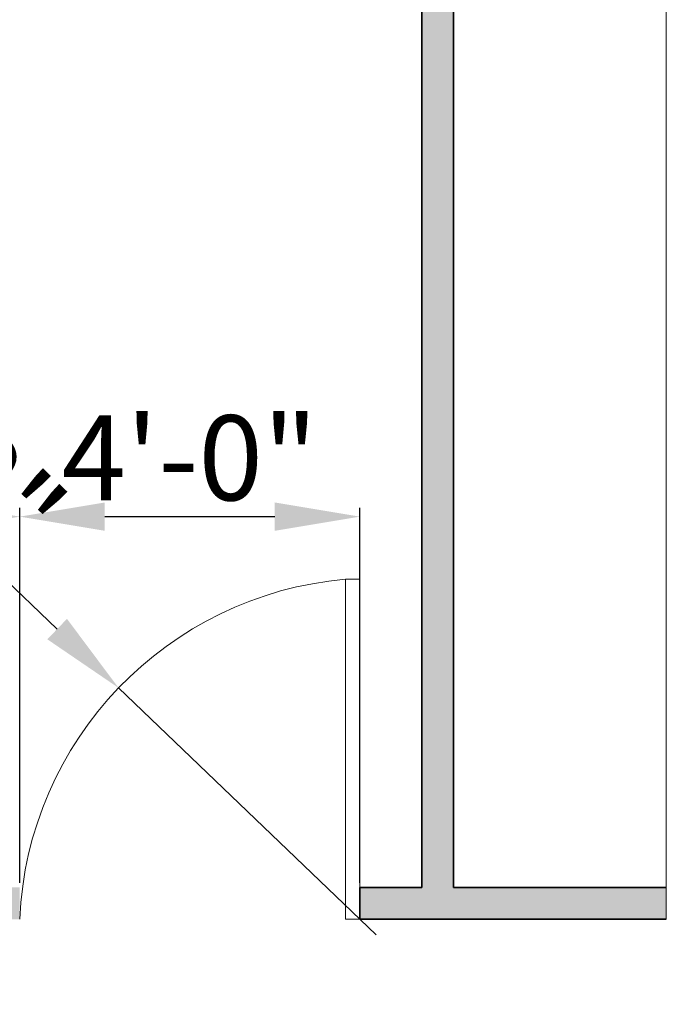
# Model space of a CAD drawing. Units: inches. Extents: x 2083 to 3317, y 1141 to 2115.
# Tile 103 of 256: x 2415 to 2508, y 1794 to 1933. Entities that reach past the tile are written whole.
import ezdxf

# ---------------------------------------------------------------- set-up
doc = ezdxf.new("R2010")
doc.units = ezdxf.units.IN
for name, color, linetype, lineweight in [('A-ANNO-DIMS', 2, 'Continuous', 18), ('A-DOOR', 4, 'Continuous', 18), ('A-FLOR-CASE', 8, 'Continuous', 18), ('A-WALL', 7, 'Continuous', 35)]:
    doc.layers.add(name, color=color, linetype=linetype, lineweight=lineweight)
doc.layers.add('A-WALL-PATT', color=251, linetype='Continuous', lineweight=13, true_color=0x636466)
doc.styles.get("Standard").update_dxf_attribs({"font": 'arial.ttf'})
doc.dimstyles.new('ISO-25', dxfattribs={"dimtxt": 12, "dimasz": 12, "dimexe": 1.25, "dimexo": 0.625, "dimtad": 1, "dimlunit": 3, "dimtxsty": 'Standard', "dimcen": 2.5, "dimadec": 0, "dimazin": 0, "dimtfac": 1, "dimtmove": 0, "dimatfit": 3, "dimfxl": 1, "dimarcsym": 0})

# ---------------------------------------------------------------- blocks, each defined once
blk = doc.blocks.new('*D53')
at = {"layer": 'A-ANNO-DIMS', "color": 0, "lineweight": -2, "transparency": 16777216}
for p, q in [((2235.96, 1810.64), (2235.96, 1863.61)), ((2414.72, 1810.64), (2414.72, 1863.61)), ((2247.96, 1862.36), (2402.72, 1862.36))]:
    blk.add_line(p, q, dxfattribs=at)
at = {"layer": 'A-ANNO-DIMS', "color": 0, "transparency": 16777216}
for points in [[(2247.96, 1864.36), (2247.96, 1860.36), (2235.96, 1862.36)], [(2402.72, 1864.36), (2402.72, 1860.36), (2414.72, 1862.36)]]:
    blk.add_solid(points, dxfattribs=at)
at = {"layer": 'Defpoints', "color": 0, "transparency": 16777216}
for p in [(2414.72, 1862.36), (2235.96, 1810.01), (2414.72, 1810.01)]:
    blk.add_point(p, dxfattribs=at)
at = {"layer": 'A-ANNO-DIMS', "color": 0, "transparency": 16777216, "insert": (2325.34, 1869.01), "char_height": 12, "attachment_point": 5}
blk.add_mtext('14\'-11"', dxfattribs=at)
blk = doc.blocks.new('*D54')
at = {"layer": 'A-ANNO-DIMS', "color": 0, "lineweight": -2, "transparency": 16777216}
for p, q in [((2414.72, 1810.64), (2414.72, 1863.61)), ((2462.72, 1810.64), (2462.72, 1863.61)), ((2426.72, 1862.36), (2450.72, 1862.36))]:
    blk.add_line(p, q, dxfattribs=at)
at = {"layer": 'A-ANNO-DIMS', "color": 0, "transparency": 16777216}
for points in [[(2426.72, 1864.36), (2426.72, 1860.36), (2414.72, 1862.36)], [(2450.72, 1864.36), (2450.72, 1860.36), (2462.72, 1862.36)]]:
    blk.add_solid(points, dxfattribs=at)
at = {"layer": 'Defpoints', "color": 0, "transparency": 16777216}
for p in [(2462.72, 1862.36), (2414.72, 1810.01), (2462.72, 1810.01)]:
    blk.add_point(p, dxfattribs=at)
at = {"layer": 'A-ANNO-DIMS', "color": 0, "transparency": 16777216, "insert": (2438.72, 1869.11), "char_height": 12, "attachment_point": 5}
blk.add_mtext('4\'-0"', dxfattribs=at)
blk = doc.blocks.new('*D68')
at = {"layer": 'A-ANNO-DIMS', "color": 0, "lineweight": -2, "transparency": 16777216}
for p, q in [((2358.93, 1905.02), (2420.01, 1846.48)), ((2465.03, 1803.34), (2428.67, 1838.18))]:
    blk.add_line(p, q, dxfattribs=at)
at = {"layer": 'A-ANNO-DIMS', "color": 0, "transparency": 16777216}
blk.add_solid([(2421.39, 1847.93), (2418.62, 1845.04), (2428.67, 1838.18)], dxfattribs=at)
at = {"layer": 'Defpoints', "color": 0, "transparency": 16777216}
for p in [(2428.67, 1838.18), (2465.03, 1803.34)]:
    blk.add_point(p, dxfattribs=at)
at = {"layer": 'A-ANNO-DIMS', "color": 0, "transparency": 16777216, "insert": (2389.86, 1884.83), "char_height": 12, "attachment_point": 5, "rotation": 316.2184}
blk.add_mtext('R4\'-2 1/2"', dxfattribs=at)

msp = doc.modelspace()

# ---------------------------------------------------------------- hatches: boundary and pattern name
at = {"layer": 'A-WALL-PATT'}
h = msp.add_hatch(color=256, dxfattribs=at)
h.dxf.hatch_style = 1
h.paths.add_polyline_path([(3126.96, 2020.761), (2748.96, 2020.761), (2604.96, 2020.761), (2226.96, 2020.761), (2226.96, 1702.761), (2466.96, 1702.761), (2466.96, 1582.761), (2418.96, 1582.761), (2418.96, 1477.761), (2226.96, 1477.761), (2226.96, 1263.261), (2544.96, 1263.261), (2544.96, 1411.761), (2604.96, 1411.761), (2685.96, 1411.761), (2685.96, 1420.761), (2604.96, 1420.761), (2604.96, 1573.761), (2604.96, 1702.761), (2604.96, 2011.761), (2748.96, 2011.761), (2748.96, 1702.761), (2862.96, 1702.761), (2862.96, 1621.761), (2871.96, 1621.761), (2871.96, 1702.761), (2883.96, 1702.761), (2883.96, 1706.939, -0.0264593), (2883.96, 1711.761), (2757.96, 1711.761), (2757.96, 1807.761), (2787.96, 1807.761), (2787.96, 1812.261), (2757.96, 1812.261), (2757.96, 2011.761), (2877.96, 2011.761), (2877.96, 1812.261), (2847.96, 1812.261), (2847.96, 1807.761), (2889.836, 1807.761), (2889.836, 1812.261), (2882.46, 1812.261), (2882.46, 2011.761), (3117.96, 2011.761), (3117.96, 1812.261), (2937.836, 1812.261), (2937.836, 1807.761), (2995.71, 1807.761), (2995.71, 1796.118), (3000.21, 1796.118), (3000.21, 1807.761), (3117.96, 1807.761), (3117.96, 1711.761), (3000.21, 1711.761), (3000.21, 1760.118), (2998.573, 1760.118, -0.020711), (2995.71, 1760.118), (2995.71, 1711.761), (2931.96, 1711.761), (2931.96, 1702.761), (3126.96, 1702.761)])
h.paths.add_polyline_path([(2471.46, 2011.761), (2471.46, 1810.011), (2462.717, 1810.011), (2462.717, 1805.511), (2505.96, 1805.511), (2505.96, 1810.011), (2475.96, 1810.011), (2475.96, 2011.761), (2595.96, 2011.761), (2595.96, 1810.011), (2565.96, 1810.011), (2565.96, 1805.511), (2595.96, 1805.511), (2595.96, 1711.761), (2235.96, 1711.761), (2235.96, 1805.511), (2353.71, 1805.511), (2353.71, 1796.054), (2358.21, 1796.054), (2358.21, 1805.511), (2414.717, 1805.511), (2414.717, 1810.011), (2235.96, 1810.011), (2235.96, 2011.761)], flags=16)
h.paths.add_polyline_path([(2270.205, 1994.61), (2270.205, 1970.61), (2246.205, 1970.61), (2246.205, 1994.61)], flags=0)
edge = h.paths.add_edge_path(flags=0)
edge.add_ellipse((2332.027, 1899.798), major_axis=(-3.043, 3.043), ratio=0.1682525, start_angle=-161.33217, end_angle=-156.30711, ccw=False)
edge.add_ellipse((2333.082, 1898.744), major_axis=(-1.055, 1.055), ratio=0.4535321, start_angle=-123.37102, end_angle=-94.15911)
edge = h.paths.add_edge_path(flags=0)
edge.add_ellipse((2332.027, 1968.876), major_axis=(3.043, 3.043), ratio=0.1682525, start_angle=18.66783, end_angle=23.69289)
edge.add_spline(control_points=[(2332.926, 1970.691), (2332.227, 1970.336), (2330.894, 1969.659), (2328.413, 1970.932), (2327.204, 1967.749), (2324.71, 1969.956), (2322.533, 1967.012), (2320.013, 1971.296), (2317.68, 1968.158), (2316.041, 1967.102), (2315.427, 1966.81)], knot_values=[0, 0, 0, 0, 2.2670587, 4.3245589, 6.6855835, 8.8786411, 11.121502, 14.300359, 17.7552837, 19.732645, 19.732645, 19.732645, 19.732645], degree=3, periodic=0)
edge.add_ellipse((2332.027, 1968.876), major_axis=(3.043, 3.043), ratio=0.1682525, start_angle=18.66783, end_angle=23.69289, ccw=False)
edge.add_ellipse((2333.082, 1969.931), major_axis=(1.055, 1.055), ratio=0.4535321, start_angle=56.62898, end_angle=85.84089, ccw=False)
edge = h.paths.add_edge_path(flags=0)
edge.add_spline(control_points=[(2296.428, 1967.988), (2293.628, 1965.336), (2287.704, 1959.727), (2299.744, 1949.996), (2294.533, 1935.669), (2290.573, 1920.604), (2293.394, 1909.974), (2296.185, 1904.967)], knot_values=[0.0991853, 0.0991853, 0.0991853, 0.0991853, 0.3453009, 0.6198217, 0.9826526, 1.3860932, 1.8105546, 1.8105546, 1.8105546, 1.8105546], degree=3, periodic=0)
edge.add_spline(control_points=[(2296.185, 1904.967), (2297.384, 1902.619), (2298.001, 1901.949), (2298.553, 1901.468)], knot_values=[0.0062457, 0.0062457, 0.0062457, 0.0062457, 0.0554759, 0.0554759, 0.0554759, 0.0554759], degree=3, periodic=0)
edge.add_spline(control_points=[(2298.553, 1901.468), (2297.259, 1900.923), (2295.225, 1900.232), (2293.06, 1900.614), (2292.101, 1900.788), (2292.09, 1900.791)], knot_values=[0.3128349, 0.3128349, 0.3128349, 0.3128349, 0.4017797, 0.4749867, 0.4759027, 0.4759027, 0.4759027, 0.4759027], degree=3, periodic=0)
edge.add_arc((2292.794, 1904.664), 3.937, 215.4209, 259.69818, ccw=False)
edge.add_spline(control_points=[(2289.585, 1902.382), (2289.477, 1902.535), (2289.368, 1902.688), (2289.261, 1902.841)], knot_values=[0.1028719, 0.1028719, 0.1028719, 0.1028719, 0.1168958, 0.1168958, 0.1168958, 0.1168958], degree=3, periodic=0)
edge.add_spline(control_points=[(2289.261, 1902.841), (2288.687, 1902.55), (2287.64, 1902.02), (2285.881, 1901.874), (2283.853, 1901.504), (2281.72, 1899.711), (2278.467, 1899.493), (2276.157, 1901.883), (2272.259, 1899.804), (2267.778, 1901.843), (2262.244, 1900.184), (2257.415, 1901.782), (2254.318, 1900.726), (2253.178, 1900.337)], knot_values=[0, 0, 0, 0, 1.9079767, 3.4771759, 5.261074, 7.9728515, 11.6802485, 13.7179214, 16.9395917, 22.789562, 27.5025027, 33.5952153, 37.1456181, 37.1456181, 37.1456181, 37.1456181], degree=3, periodic=0)
edge.add_line((2253.178, 1900.337), (2250.244, 1902.841))
edge.add_line((2250.244, 1902.841), (2250.244, 1965.833))
edge.add_line((2250.244, 1965.833), (2253.178, 1968.337))
edge.add_spline(control_points=[(2253.178, 1968.337), (2254.318, 1967.948), (2257.415, 1966.892), (2262.244, 1968.49), (2267.778, 1966.831), (2271.527, 1968.537), (2273.876, 1967.828), (2274.207, 1967.728)], knot_values=[0, 0, 0, 0, 0.0901802, 0.2449351, 0.3646438, 0.5132331, 0.5378548, 0.5378548, 0.5378548, 0.5378548], degree=3, periodic=0)
edge.add_arc((2274.353, 1963.793), 3.937, 72.05113, 92.12795, ccw=False)
edge.add_arc((2281.297, 1985.23), 18.596, 252.05113, 288.56572)
edge.add_arc((2292.317, 1956.029), 12.646, 71.02679, 113.77822, ccw=False)
edge = h.paths.add_edge_path(flags=0)
edge.add_spline(control_points=[(2274.899, 1951.856), (2275.066, 1951.617), (2275.233, 1951.377), (2275.398, 1951.136)], knot_values=[1.4099157, 1.4099157, 1.4099157, 1.4099157, 1.4315903, 1.4315903, 1.4315903, 1.4315903], degree=3, periodic=0)
edge.add_spline(control_points=[(2275.398, 1951.136), (2275.792, 1950.562), (2276.179, 1949.984), (2276.546, 1949.397)], knot_values=[1.3582378, 1.3582378, 1.3582378, 1.3582378, 1.4099157, 1.4099157, 1.4099157, 1.4099157], degree=3, periodic=0)
edge.add_line((2276.546, 1949.397), (2277.437, 1947.862))
edge.add_spline(control_points=[(2277.437, 1947.862), (2276.304, 1945.673), (2274.64, 1942.427), (2274.632, 1938.094), (2272.799, 1930.852), (2274.356, 1943.897), (2275.948, 1947.923), (2276.546, 1949.397)], knot_values=[0.0056315, 0.0056315, 0.0056315, 0.0056315, 0.1860139, 0.2660015, 0.3570872, 0.5963902, 0.7397317, 0.7397317, 0.7397317, 0.7397317], degree=3, periodic=0)
edge.add_spline(control_points=[(2276.546, 1949.397), (2276.179, 1949.984), (2275.792, 1950.562), (2275.398, 1951.136)], knot_values=[1.3582378, 1.3582378, 1.3582378, 1.3582378, 1.4099157, 1.4099157, 1.4099157, 1.4099157], degree=3, periodic=0)
edge.add_spline(control_points=[(2275.398, 1951.136), (2274.943, 1950.08), (2274.208, 1948.025), (2273.935, 1944.851), (2272.469, 1937.627), (2273.466, 1945.696), (2274.701, 1951.059), (2274.899, 1951.856)], knot_values=[0.1043639, 0.1043639, 0.1043639, 0.1043639, 0.1896363, 0.2696239, 0.3607096, 0.6000126, 0.6446217, 0.6446217, 0.6446217, 0.6446217], degree=3, periodic=0)
h.paths.add_polyline_path([(2269.168, 1963.128, -0.3575267), (2268.171, 1960.976, -0.0925607), (2268.171, 1939.436, -0.3575267), (2269.168, 1937.285, -0.3575267), (2267.016, 1938.282, -0.1647847), (2254.686, 1938.282, -0.3575267), (2252.534, 1937.285, -0.3575267), (2253.531, 1939.436, -0.0925607), (2253.531, 1960.976, -0.3575267), (2252.534, 1963.128, -0.3575267), (2254.686, 1962.131, -0.1647847), (2267.016, 1962.131, -0.3575267)], flags=0)
h.paths.add_polyline_path([(2248.874, 1967.802), (2248.874, 1957.028), (2249.458, 1957.028), (2249.458, 1911.647), (2248.874, 1911.647), (2248.874, 1900.873), (2246.512, 1900.873, 0.1973271), (2244.15, 1902.457), (2244.15, 1966.218, 0.1973271), (2246.512, 1967.802)], flags=0)
h.paths.add_polyline_path([(2269.168, 1931.389, -0.3575267), (2268.171, 1929.238, -0.0925607), (2268.171, 1907.698, -0.3575267), (2269.168, 1905.547, -0.3575267), (2267.016, 1906.544, -0.1647847), (2254.686, 1906.544, -0.3575267), (2252.534, 1905.547, -0.3575267), (2253.531, 1907.698, -0.0925607), (2253.531, 1929.238, -0.3575267), (2252.534, 1931.389, -0.3575267), (2254.686, 1930.392, -0.1647847), (2267.016, 1930.392, -0.3575267)], flags=0)
edge = h.paths.add_edge_path(flags=0)
edge.add_spline(control_points=[(2276.197, 1906.724), (2276.168, 1909.029), (2276.114, 1913.372), (2270.598, 1924.925), (2273.905, 1919.013), (2275.922, 1916.262), (2275.475, 1912.402), (2277.258, 1910.381), (2276.696, 1908.225), (2276.646, 1906.813), (2276.618, 1906.008)], knot_values=[0, 0, 0, 0, 8.6102597, 16.2212739, 18.8430575, 23.8048978, 27.4408283, 29.3561016, 31.2034776, 33.6506866, 33.6506866, 33.6506866, 33.6506866], degree=3, periodic=0)
edge.add_spline(control_points=[(2276.618, 1906.008), (2276.623, 1905.624), (2276.498, 1904.629), (2275.442, 1903.855), (2274.937, 1903.08), (2274.859, 1902.841)], knot_values=[0.1564884, 0.1564884, 0.1564884, 0.1564884, 0.1843975, 0.2313765, 0.2505985, 0.2505985, 0.2505985, 0.2505985], degree=3, periodic=0)
edge.add_line((2274.859, 1902.841), (2276.506, 1902.841))
edge.add_spline(control_points=[(2276.506, 1902.841), (2276.788, 1903.085), (2277.665, 1904.125), (2278.25, 1904.341), (2277.654, 1908.527), (2278.156, 1906.228), (2278.1, 1905.286), (2278.847, 1904.069), (2277.857, 1903.415), (2277.874, 1902.991), (2277.904, 1902.841)], knot_values=[0.0595743, 0.0595743, 0.0595743, 0.0595743, 0.0807529, 0.1037415, 0.1697201, 0.1760361, 0.2071372, 0.2404744, 0.2623409, 0.2736605, 0.2736605, 0.2736605, 0.2736605], degree=3, periodic=0)
edge.add_line((2277.904, 1902.841), (2280.03, 1902.841))
edge.add_spline(control_points=[(2280.03, 1902.841), (2279.888, 1903.088), (2279.499, 1903.982), (2280.152, 1905.939), (2278.104, 1909.658), (2279.762, 1907.185), (2280.328, 1904.875), (2280.485, 1903.49), (2281.463, 1903.249), (2281.758, 1902.936), (2281.834, 1902.841)], knot_values=[0.013856, 0.013856, 0.013856, 0.013856, 0.0348738, 0.0888667, 0.1078792, 0.1267378, 0.158714, 0.1937575, 0.2174868, 0.2267221, 0.2267221, 0.2267221, 0.2267221], degree=3, periodic=0)
edge.add_spline(control_points=[(2281.834, 1902.841), (2281.788, 1902.827), (2281.647, 1902.783), (2281.396, 1902.859), (2281.088, 1902.985), (2280.721, 1903.061), (2280.333, 1903.026), (2280.125, 1902.899), (2280.03, 1902.841)], knot_values=[0, 0, 0, 0, 0.1441304, 0.435517, 0.7492759, 1.1530457, 1.5483707, 1.878348, 1.878348, 1.878348, 1.878348], degree=3, periodic=0)
edge.add_line((2280.03, 1902.841), (2277.904, 1902.841))
edge.add_spline(control_points=[(2277.904, 1902.841), (2277.893, 1902.796), (2277.865, 1902.68), (2277.607, 1902.687), (2277.274, 1902.801), (2276.838, 1902.62), (2276.584, 1902.789), (2276.506, 1902.841)], knot_values=[0, 0, 0, 0, 0.1271885, 0.3261988, 0.6280094, 1.2435704, 1.5153306, 1.5153306, 1.5153306, 1.5153306], degree=3, periodic=0)
edge.add_line((2276.506, 1902.841), (2274.859, 1902.841))
edge.add_spline(control_points=[(2274.859, 1902.841), (2274.814, 1902.899), (2274.725, 1903.013), (2274.493, 1903.119), (2274.244, 1902.961), (2273.937, 1903.185), (2273.614, 1902.983), (2273.408, 1902.883), (2273.322, 1902.841)], knot_values=[0, 0, 0, 0, 0.2184302, 0.4369566, 0.6879766, 0.9903786, 1.3983955, 1.6918498, 1.6918498, 1.6918498, 1.6918498], degree=3, periodic=0)
edge.add_spline(control_points=[(2273.322, 1902.841), (2273.617, 1903.446), (2274.274, 1904.538), (2276.027, 1904.574), (2276.207, 1906.584), (2276.197, 1906.724)], knot_values=[0.0122268, 0.0122268, 0.0122268, 0.0122268, 0.0594721, 0.1062177, 0.134458, 0.134458, 0.134458, 0.134458], degree=3, periodic=0)
h.paths.add_polyline_path([(2270.776, 1897.79), (2270.776, 1873.79), (2246.776, 1873.79), (2246.776, 1897.79)], flags=0)
h.paths.add_polyline_path([(2353.71, 1760.005), (2353.71, 1760.054), (2358.21, 1760.054, -0.033729)], flags=0)
h.paths.add_polyline_path([(2321.819, 1737.529), (2341.995, 1737.529, -0.4142136), (2343.203, 1736.321), (2343.203, 1721.021, -0.4142136), (2341.995, 1719.813), (2321.819, 1719.813, -0.4142136), (2320.611, 1721.021), (2320.611, 1736.321, -0.4142136)], flags=0)
h.paths.add_polyline_path([(2324.235, 1736.321), (2339.579, 1736.321, -0.4142136), (2341.995, 1733.905), (2341.995, 1725.45, -0.4142136), (2339.579, 1723.034), (2333.681, 1723.034), (2333.845, 1722.045, -0.8706461), (2335.425, 1721.826, -0.767327), (2333.923, 1721.423), (2331.291, 1721.423, -0.767327), (2329.788, 1721.826, -0.8706461), (2331.368, 1722.045), (2331.533, 1723.034), (2324.235, 1723.034, -0.4142136), (2321.819, 1725.45), (2321.819, 1733.905, -0.4142136)], flags=0)
h.paths.add_polyline_path([(2570.484, 1928.615), (2589.684, 1928.615), (2590.169, 1928.615), (2590.169, 1904.993), (2570.484, 1904.993)], flags=0)
h.paths.add_polyline_path([(2574.447, 1927.264, -1), (2572.829, 1927.264, -1)], flags=0)
h.paths.add_polyline_path([(2573.09, 1926.941), (2573.925, 1927.776), (2574.148, 1927.553), (2573.313, 1926.718)], flags=0)
h.paths.add_polyline_path([(2578.779, 1919.73, -1), (2571.592, 1919.73, -1)], flags=0)
h.paths.add_polyline_path([(2578.385, 1919.73, -1), (2571.985, 1919.73, -1)], flags=0)
h.paths.add_polyline_path([(2331.596, 1729.476, -1), (2333.618, 1729.476, -1)], flags=0)
h.paths.add_polyline_path([(2578.034, 1927.264, -1), (2576.416, 1927.264, -1)], flags=0)
h.paths.add_polyline_path([(2576.689, 1927.531), (2576.912, 1927.754), (2577.747, 1926.919), (2577.524, 1926.696)], flags=0)
h.paths.add_polyline_path([(2578.139, 1909.86, -1), (2572.232, 1909.86, -1)], flags=0)
h.paths.add_polyline_path([(2577.745, 1909.86, -1), (2572.625, 1909.86, -1)], flags=0)
h.paths.add_polyline_path([(2583.798, 1927.264, -1), (2582.179, 1927.264, -1)], flags=0)
h.paths.add_polyline_path([(2582.719, 1927.754), (2583.554, 1926.919), (2583.331, 1926.696), (2582.496, 1927.531)], flags=0)
h.paths.add_polyline_path([(2582.496, 1927.531), (2582.719, 1927.754), (2583.554, 1926.919), (2583.331, 1926.696)], flags=0)
h.paths.add_polyline_path([(2587.739, 1920.53, -1), (2581.832, 1920.53, -1)], flags=0)
h.paths.add_polyline_path([(2587.345, 1920.53, -1), (2582.225, 1920.53, -1)], flags=0)
h.paths.add_polyline_path([(2587.385, 1927.264, -1), (2585.766, 1927.264, -1)], flags=0)
h.paths.add_polyline_path([(2586.082, 1926.98), (2586.917, 1927.815), (2587.14, 1927.593), (2586.305, 1926.758)], flags=0)
h.paths.add_polyline_path([(2588.379, 1910.66, -1), (2581.192, 1910.66, -1)], flags=0)
h.paths.add_polyline_path([(2587.985, 1910.66, -1), (2581.585, 1910.66, -1)], flags=0)
h.paths.add_polyline_path([(2417.168, 1729.478), (2437.344, 1729.478, -0.4142136), (2438.552, 1728.27), (2438.552, 1712.969, -0.4142136), (2437.344, 1711.761), (2417.168, 1711.761, -0.4142136), (2415.96, 1712.969), (2415.96, 1728.27, -0.4142136)], flags=0)
h.paths.add_polyline_path([(2419.584, 1728.27), (2434.928, 1728.27, -0.4142136), (2437.344, 1725.854), (2437.344, 1717.398, -0.4142136), (2434.928, 1714.983), (2429.029, 1714.983), (2429.194, 1713.994, -0.8706461), (2430.774, 1713.775, -0.767327), (2429.271, 1713.372), (2426.64, 1713.372, -0.767327), (2425.137, 1713.775, -0.8706461), (2426.717, 1713.994), (2426.882, 1714.983), (2419.584, 1714.983, -0.4142136), (2417.168, 1717.398), (2417.168, 1725.854, -0.4142136)], flags=0)
h.paths.add_polyline_path([(2419.584, 1728.27), (2434.928, 1728.27, -0.4142136), (2437.344, 1725.854), (2437.344, 1717.398, -0.4142136), (2434.928, 1714.983), (2429.029, 1714.983), (2428.358, 1719.009), (2427.553, 1719.009), (2426.882, 1714.983), (2419.584, 1714.983, -0.4142136), (2417.168, 1717.398), (2417.168, 1725.854, -0.4142136)], flags=0)
h.paths.add_polyline_path([(2426.944, 1721.425, -1), (2428.967, 1721.425, -1)], flags=0)
h.paths.add_polyline_path([(2475.96, 1702.761), (2595.96, 1702.761), (2595.96, 1582.761), (2475.96, 1582.761)], flags=16)
h.paths.add_polyline_path([(2427.96, 1573.761), (2595.96, 1573.761), (2595.96, 1468.761), (2595.96, 1420.761), (2384.46, 1420.761), (2384.46, 1468.761), (2427.96, 1468.761)], flags=16)
h.paths.add_polyline_path([(2379.96, 1468.761), (2379.96, 1420.761), (2235.96, 1420.761), (2235.96, 1468.761)], flags=16)
h.paths.add_polyline_path([(2317.816, 1466.696), (2337.992, 1466.696, -0.4142136), (2339.2, 1465.488), (2339.2, 1450.187, -0.4142136), (2337.992, 1448.979), (2317.816, 1448.979, -0.4142136), (2316.608, 1450.187), (2316.608, 1465.488, -0.4142136)], flags=0)
h.paths.add_polyline_path([(2320.232, 1465.488), (2335.576, 1465.488, -0.4142136), (2337.992, 1463.072), (2337.992, 1454.616, -0.4142136), (2335.576, 1452.2), (2329.677, 1452.2), (2329.842, 1451.212, -0.8706461), (2331.422, 1450.992, -0.767327), (2329.92, 1450.59), (2327.288, 1450.59, -0.767327), (2325.785, 1450.992, -0.8706461), (2327.365, 1451.212), (2327.53, 1452.2), (2320.232, 1452.2, -0.4142136), (2317.816, 1454.616), (2317.816, 1463.072, -0.4142136)], flags=0)
h.paths.add_polyline_path([(2320.232, 1465.488), (2335.576, 1465.488, -0.4142136), (2337.992, 1463.072), (2337.992, 1454.616, -0.4142136), (2335.576, 1452.2), (2329.677, 1452.2), (2329.006, 1456.227), (2328.201, 1456.227), (2327.53, 1452.2), (2320.232, 1452.2, -0.4142136), (2317.816, 1454.616), (2317.816, 1463.072, -0.4142136)], flags=0)
h.paths.add_polyline_path([(2327.593, 1458.643, -1), (2329.615, 1458.643, -1)], flags=0)
h.paths.add_polyline_path([(2244.412, 1433.34), (2241.921, 1433.34, -0.4142136), (2240.018, 1435.244), (2240.018, 1440.953, -0.4142105), (2241.921, 1442.856), (2244.412, 1442.856, -1.9764724)], flags=0)
h.paths.add_polyline_path([(2245.357, 1434.398, -0.4142136), (2245.357, 1441.799, -2.1440985)], flags=0)
h.paths.add_polyline_path([(2535.96, 1416.261), (2535.96, 1272.261), (2235.96, 1272.261), (2235.96, 1416.261)], flags=16)
h.paths.add_polyline_path([(2260.12, 1384.293), (2260.12, 1362.039), (2237.865, 1362.039), (2237.865, 1384.293)], flags=0)
edge = h.paths.add_edge_path(flags=0)
edge.add_line((2318.252, 1362.093), (2318.146, 1362.001))
edge.add_ellipse((2317.445, 1360.431), major_axis=(2.822, 2.822), ratio=0.1682525, start_angle=18.66783, end_angle=20.94813, ccw=False)
edge.add_ellipse((2318.423, 1361.409), major_axis=(0.978, 0.978), ratio=0.4535321, start_angle=56.62898, end_angle=70.2262, ccw=False)
edge = h.paths.add_edge_path(flags=0)
edge.add_line((2319.107, 1295.571), (2319.015, 1295.677))
edge.add_ellipse((2317.445, 1296.378), major_axis=(-2.822, 2.822), ratio=0.1682525, start_angle=-161.33217, end_angle=-159.05187, ccw=False)
edge.add_ellipse((2318.423, 1295.4), major_axis=(-0.978, 0.978), ratio=0.4535321, start_angle=-123.37102, end_angle=-109.7738)
edge = h.paths.add_edge_path(flags=0)
edge.add_spline(control_points=[(2284.21, 1301.17), (2284.581, 1300.445), (2284.891, 1299.892), (2285.16, 1299.461)], knot_values=[0.0390658, 0.0390658, 0.0390658, 0.0390658, 0.0554759, 0.0554759, 0.0554759, 0.0554759], degree=3, periodic=0)
edge.add_line((2285.16, 1299.461), (2284.21, 1301.17))
edge = h.paths.add_edge_path(flags=0)
edge.add_line((2280.412, 1297.298), (2283.37, 1297.036))
edge.add_line((2283.37, 1297.036), (2286.406, 1297.926))
edge.add_spline(control_points=[(2286.406, 1297.926), (2285.305, 1297.463), (2284.345, 1297.129), (2283.37, 1297.036)], knot_values=[0.3943688, 0.3943688, 0.3943688, 0.3943688, 0.4759027, 0.4759027, 0.4759027, 0.4759027], degree=3, periodic=0)
edge.add_spline(control_points=[(2283.37, 1297.036), (2283.281, 1297.028), (2282.316, 1296.957), (2281.313, 1297.134), (2280.423, 1297.296), (2280.412, 1297.298)], knot_values=[0.3128349, 0.3128349, 0.3128349, 0.3128349, 0.3202458, 0.3934528, 0.3943688, 0.3943688, 0.3943688, 0.3943688], degree=3, periodic=0)
edge = h.paths.add_edge_path(flags=0)
edge.add_line((2284.436, 1359.607), (2280.446, 1355.328))
edge.add_line((2280.446, 1355.328), (2279.58, 1351.018))
edge.add_line((2279.58, 1351.018), (2282.413, 1346.58))
edge.add_spline(control_points=[(2282.413, 1346.58), (2283.153, 1345.589), (2284.253, 1344.029), (2284.801, 1342.387), (2284.935, 1341.806)], knot_values=[1.2400982, 1.2400982, 1.2400982, 1.2400982, 1.3328922, 1.3827123, 1.3827123, 1.3827123, 1.3827123], degree=3, periodic=0)
edge.add_spline(control_points=[(2284.935, 1341.806), (2285.319, 1340.141), (2285.233, 1338.409), (2284.91, 1336.654)], knot_values=[1.0974841, 1.0974841, 1.0974841, 1.0974841, 1.2400982, 1.2400982, 1.2400982, 1.2400982], degree=3, periodic=0)
edge.add_spline(control_points=[(2284.91, 1336.654), (2284.587, 1334.899), (2284.027, 1333.12), (2283.463, 1331.361)], knot_values=[0.9548699, 0.9548699, 0.9548699, 0.9548699, 1.0974841, 1.0974841, 1.0974841, 1.0974841], degree=3, periodic=0)
edge.add_line((2283.463, 1331.361), (2281.89, 1326.153))
edge.add_line((2281.89, 1326.153), (2280.756, 1321.056))
edge.add_line((2280.756, 1321.056), (2280.299, 1316.002))
edge.add_line((2280.299, 1316.002), (2280.716, 1310.95))
edge.add_line((2280.716, 1310.95), (2282.028, 1305.972))
edge.add_line((2282.028, 1305.972), (2284.21, 1301.17))
edge.add_spline(control_points=[(2284.21, 1301.17), (2283.341, 1302.73), (2282.612, 1304.336), (2282.028, 1305.972)], knot_values=[0.0991853, 0.0991853, 0.0991853, 0.0991853, 0.2417994, 0.2417994, 0.2417994, 0.2417994], degree=3, periodic=0)
edge.add_spline(control_points=[(2282.028, 1305.972), (2281.444, 1307.608), (2281.005, 1309.273), (2280.716, 1310.95)], knot_values=[0.2417994, 0.2417994, 0.2417994, 0.2417994, 0.3844135, 0.3844135, 0.3844135, 0.3844135], degree=3, periodic=0)
edge.add_spline(control_points=[(2280.716, 1310.95), (2280.433, 1312.588), (2280.289, 1314.277), (2280.299, 1315.962), (2280.299, 1316.002)], knot_values=[0.3844135, 0.3844135, 0.3844135, 0.3844135, 0.5236467, 0.5270276, 0.5270276, 0.5270276, 0.5270276], degree=3, periodic=0)
edge.add_spline(control_points=[(2280.299, 1316.002), (2280.312, 1317.687), (2280.478, 1319.368), (2280.756, 1321.056)], knot_values=[0.5270276, 0.5270276, 0.5270276, 0.5270276, 0.6696417, 0.6696417, 0.6696417, 0.6696417], degree=3, periodic=0)
edge.add_spline(control_points=[(2280.756, 1321.056), (2281.035, 1322.744), (2281.426, 1324.44), (2281.89, 1326.153)], knot_values=[0.6696417, 0.6696417, 0.6696417, 0.6696417, 0.8122558, 0.8122558, 0.8122558, 0.8122558], degree=3, periodic=0)
edge.add_spline(control_points=[(2281.89, 1326.153), (2282.264, 1327.533), (2282.788, 1329.262), (2283.353, 1331.018), (2283.463, 1331.361)], knot_values=[0.8122558, 0.8122558, 0.8122558, 0.8122558, 0.9270873, 0.9548699, 0.9548699, 0.9548699, 0.9548699], degree=3, periodic=0)
edge.add_line((2283.463, 1331.361), (2284.91, 1336.654))
edge.add_line((2284.91, 1336.654), (2284.935, 1341.806))
edge.add_line((2284.935, 1341.806), (2282.413, 1346.58))
edge.add_spline(control_points=[(2282.413, 1346.58), (2281.275, 1348.104), (2280.078, 1349.57), (2279.58, 1351.018)], knot_values=[1.3827123, 1.3827123, 1.3827123, 1.3827123, 1.5253264, 1.5253264, 1.5253264, 1.5253264], degree=3, periodic=0)
edge.add_spline(control_points=[(2279.58, 1351.018), (2279.443, 1351.415), (2279.136, 1352.857), (2279.735, 1354.29), (2280.446, 1355.328)], knot_values=[1.5253264, 1.5253264, 1.5253264, 1.5253264, 1.564439, 1.6679405, 1.6679405, 1.6679405, 1.6679405], degree=3, periodic=0)
edge.add_spline(control_points=[(2280.446, 1355.328), (2281.426, 1356.758), (2282.931, 1358.183), (2284.436, 1359.607)], knot_values=[1.6679405, 1.6679405, 1.6679405, 1.6679405, 1.8105546, 1.8105546, 1.8105546, 1.8105546], degree=3, periodic=0)
edge.add_arc((2280.623, 1348.518), 11.726, 71.02679, 113.77822)
edge.add_arc((2270.405, 1375.595), 17.244, 252.05113, 288.56572, ccw=False)
edge.add_arc((2263.966, 1355.718), 3.651, 72.05113, 92.12795)
edge.add_arc((2263.966, 1355.718), 3.651, 92.12795, 177.98513)
edge.add_spline(control_points=[(2260.318, 1355.846), (2260.26, 1354.221), (2260.551, 1350.187), (2262.999, 1346.766), (2264.473, 1344.649)], knot_values=[1.4315903, 1.4315903, 1.4315903, 1.4315903, 1.5641438, 1.7706953, 1.7706953, 1.7706953, 1.7706953], degree=3, periodic=0)
edge.add_line((2264.473, 1344.649), (2264.936, 1343.983))
edge.add_spline(control_points=[(2263.801, 1340.248), (2263.843, 1340.514), (2264.067, 1341.756), (2264.513, 1343.002), (2264.935, 1343.981)], knot_values=[0.5365702, 0.5365702, 0.5365702, 0.5365702, 0.5593494, 0.6446217, 0.6446217, 0.6446217, 0.6446217], degree=3, periodic=0)
edge.add_spline(control_points=[(2264.935, 1343.981), (2265.118, 1343.715), (2265.299, 1343.448), (2265.477, 1343.179)], knot_values=[1.3840767, 1.3840767, 1.3840767, 1.3840767, 1.4099157, 1.4099157, 1.4099157, 1.4099157], degree=3, periodic=0)
edge.add_spline(control_points=[(2265.477, 1343.179), (2265.655, 1342.911), (2265.829, 1342.641), (2265.999, 1342.369)], knot_values=[1.3582378, 1.3582378, 1.3582378, 1.3582378, 1.3840767, 1.3840767, 1.3840767, 1.3840767], degree=3, periodic=0)
edge.add_line((2265.999, 1342.369), (2266.826, 1340.946))
edge.add_spline(control_points=[(2266.826, 1340.946), (2268.894, 1337.09), (2271.398, 1325.843), (2270.516, 1310.569), (2275.919, 1301.861), (2277.79, 1299.199)], knot_values=[0.1168958, 0.1168958, 0.1168958, 0.1168958, 0.4729873, 1.0509689, 1.3137934, 1.3137934, 1.3137934, 1.3137934], degree=3, periodic=0)
edge.add_spline(control_points=[(2277.79, 1299.199), (2277.839, 1299.128), (2277.889, 1299.057), (2277.94, 1298.987)], knot_values=[0.1098839, 0.1098839, 0.1098839, 0.1098839, 0.1168958, 0.1168958, 0.1168958, 0.1168958], degree=3, periodic=0)
edge.add_line((2277.94, 1298.987), (2277.789, 1299.199))
edge.add_spline(control_points=[(2277.789, 1299.199), (2277.257, 1298.929), (2276.286, 1298.438), (2275.039, 1298.334), (2274.383, 1298.239), (2274.215, 1298.209)], knot_values=[33.1218702, 33.1218702, 33.1218702, 33.1218702, 35.0290557, 36.5982549, 37.1448269, 37.1448269, 37.1448269, 37.1448269], degree=3, periodic=0)
edge.add_line((2274.215, 1298.209), (2273.073, 1297.893))
edge.add_spline(control_points=[(2273.073, 1297.893), (2272.323, 1297.58), (2271.039, 1296.511), (2269.248, 1296.226), (2268.423, 1296.375)], knot_values=[26.5325843, 26.5325843, 26.5325843, 26.5325843, 29.198919, 31.8391012, 31.8391012, 31.8391012, 31.8391012], degree=3, periodic=0)
edge.add_line((2268.423, 1296.375), (2263.879, 1297.458))
edge.add_spline(control_points=[(2263.879, 1297.458), (2263.556, 1297.359), (2261.86, 1296.839), (2260.239, 1297.282), (2258.933, 1297.516)], knot_values=[15.9195506, 15.9195506, 15.9195506, 15.9195506, 16.9395917, 21.2260675, 21.2260675, 21.2260675, 21.2260675], degree=3, periodic=0)
edge.add_line((2258.933, 1297.516), (2254.055, 1297.329))
edge.add_spline(control_points=[(2254.055, 1297.329), (2253.756, 1297.296), (2252.114, 1297.165), (2250.462, 1297.544), (2249.13, 1297.668)], knot_values=[5.3065169, 5.3065169, 5.3065169, 5.3065169, 6.2764352, 10.6130337, 10.6130337, 10.6130337, 10.6130337], degree=3, periodic=0)
edge.add_line((2249.13, 1297.668), (2244.332, 1296.878))
edge.add_line((2244.332, 1296.878), (2241.611, 1299.199))
edge.add_line((2241.611, 1299.199), (2241.611, 1357.609))
edge.add_line((2241.611, 1357.609), (2244.332, 1359.931))
edge.add_line((2244.332, 1359.931), (2252.729, 1359.543))
edge.add_spline(control_points=[(2252.729, 1359.543), (2252.871, 1359.546), (2253.306, 1359.548), (2253.74, 1359.514), (2254.032, 1359.482)], knot_values=[0.233291, 0.233291, 0.233291, 0.233291, 0.2449351, 0.2689274, 0.2689274, 0.2689274, 0.2689274], degree=3, periodic=0)
edge.add_line((2254.032, 1359.482), (2259.587, 1359.416))
edge.add_spline(control_points=[(2259.587, 1359.416), (2260.677, 1359.629), (2262.073, 1359.897), (2263.524, 1359.459), (2263.83, 1359.366)], knot_values=[0.4225164, 0.4225164, 0.4225164, 0.4225164, 0.5132331, 0.5378548, 0.5378548, 0.5378548, 0.5378548], degree=3, periodic=0)
edge.add_arc((2263.966, 1355.718), 3.651, 72.05113, 92.12795, ccw=False)
edge.add_arc((2270.405, 1375.595), 17.244, 252.05113, 288.56572)
edge.add_arc((2280.623, 1348.518), 11.726, 71.02679, 113.77822, ccw=False)
h.paths.add_polyline_path([(2240.341, 1359.435), (2240.341, 1349.444), (2240.882, 1349.444), (2240.882, 1307.365), (2240.341, 1307.365), (2240.341, 1297.374), (2238.15, 1297.374, 0.1973271), (2235.96, 1298.843), (2235.96, 1357.966, 0.1973271), (2238.15, 1359.435)], flags=0)
h.paths.add_polyline_path([(2259.158, 1355.101, -0.3575267), (2258.233, 1353.106, -0.0925607), (2258.233, 1333.133, -0.3575267), (2259.158, 1331.138, -0.3575267), (2257.163, 1332.062, -0.1647847), (2245.729, 1332.062, -0.3575267), (2243.735, 1331.138, -0.3575267), (2244.659, 1333.133, -0.0925607), (2244.659, 1353.106, -0.3575267), (2243.735, 1355.101, -0.3575267), (2245.729, 1354.176, -0.1647847), (2257.163, 1354.176, -0.3575267)], flags=0)
edge = h.paths.add_edge_path(flags=0)
edge.add_line((2265.999, 1342.369), (2266.826, 1340.946))
edge.add_line((2266.826, 1340.946), (2265.308, 1337.814))
edge.add_line((2265.308, 1337.814), (2264.358, 1334.653))
edge.add_line((2264.358, 1334.653), (2264.262, 1333.8))
edge.add_spline(control_points=[(2264.262, 1333.8), (2264.208, 1333.187), (2264.162, 1332.366), (2264.007, 1331.414), (2263.969, 1331.202)], knot_values=[0.4644442, 0.4644442, 0.4644442, 0.4644442, 0.5166905, 0.5316081, 0.5316081, 0.5316081, 0.5316081], degree=3, periodic=0)
edge.add_spline(control_points=[(2263.969, 1331.202), (2263.775, 1330.119), (2263.424, 1328.791), (2263.257, 1328.531), (2263.234, 1328.515)], knot_values=[0.3726816, 0.3726816, 0.3726816, 0.3726816, 0.4488497, 0.4644442, 0.4644442, 0.4644442, 0.4644442], degree=3, periodic=0)
edge.add_spline(control_points=[(2263.234, 1328.515), (2263.096, 1328.42), (2263.131, 1329.301), (2263.275, 1330.616)], knot_values=[0.2809191, 0.2809191, 0.2809191, 0.2809191, 0.3726816, 0.3726816, 0.3726816, 0.3726816], degree=3, periodic=0)
edge.add_spline(control_points=[(2263.275, 1330.616), (2263.419, 1331.93), (2263.672, 1333.677), (2263.97, 1335.315)], knot_values=[0.1891566, 0.1891566, 0.1891566, 0.1891566, 0.2809191, 0.2809191, 0.2809191, 0.2809191], degree=3, periodic=0)
edge.add_spline(control_points=[(2263.97, 1335.315), (2264.1, 1336.032), (2264.419, 1337.622), (2264.755, 1338.864), (2264.947, 1339.491)], knot_values=[0.097394, 0.097394, 0.097394, 0.097394, 0.1375775, 0.1891566, 0.1891566, 0.1891566, 0.1891566], degree=3, periodic=0)
edge.add_spline(control_points=[(2264.947, 1339.491), (2265.29, 1340.606), (2265.644, 1341.494), (2265.999, 1342.369)], knot_values=[0.0056315, 0.0056315, 0.0056315, 0.0056315, 0.097394, 0.097394, 0.097394, 0.097394], degree=3, periodic=0)
h.paths.add_polyline_path([(2259.158, 1325.671, -0.3575267), (2258.233, 1323.676, -0.0925607), (2258.233, 1303.703, -0.3575267), (2259.158, 1301.708, -0.3575267), (2257.163, 1302.633, -0.1647847), (2245.729, 1302.633, -0.3575267), (2243.735, 1301.708, -0.3575267), (2244.659, 1303.703, -0.0925607), (2244.659, 1323.676, -0.3575267), (2243.735, 1325.671, -0.3575267), (2245.729, 1324.747, -0.1647847), (2257.163, 1324.747, -0.3575267)], flags=0)
edge = h.paths.add_edge_path(flags=0)
edge.add_spline(control_points=[(2261.709, 1317.311), (2261.679, 1317.418), (2261.762, 1317.389), (2262.491, 1316.09), (2262.962, 1315.301)], knot_values=[14.9558607, 14.9558607, 14.9558607, 14.9558607, 16.2212739, 18.6948259, 18.6948259, 18.6948259, 18.6948259], degree=3, periodic=0)
edge.add_spline(control_points=[(2262.962, 1315.301), (2262.99, 1315.254), (2263.702, 1314.067), (2264.349, 1313.127), (2264.73, 1312.164)], knot_values=[18.6948259, 18.6948259, 18.6948259, 18.6948259, 18.8430575, 22.433791, 22.433791, 22.433791, 22.433791], degree=3, periodic=0)
edge.add_spline(control_points=[(2264.73, 1312.164), (2264.876, 1311.796), (2265.177, 1310.77), (2265.143, 1309.559), (2265.248, 1308.824)], knot_values=[22.433791, 22.433791, 22.433791, 22.433791, 23.8048978, 26.1727562, 26.1727562, 26.1727562, 26.1727562], degree=3, periodic=0)
edge.add_line((2265.248, 1308.824), (2265.851, 1307.172))
edge.add_spline(control_points=[(2265.851, 1307.172), (2266.065, 1306.822), (2266.384, 1306.332), (2266.424, 1305.781), (2266.42, 1305.611)], knot_values=[28.0625624, 28.0625624, 28.0625624, 28.0625624, 29.3561016, 29.9117214, 29.9117214, 29.9117214, 29.9117214], degree=3, periodic=0)
edge.add_spline(control_points=[(2266.42, 1305.611), (2266.416, 1305.433), (2266.394, 1305.25), (2266.365, 1305.066)], knot_values=[29.9117214, 29.9117214, 29.9117214, 29.9117214, 30.4978371, 30.4978371, 30.4978371, 30.4978371], degree=3, periodic=0)
edge.add_line((2266.365, 1305.066), (2266.066, 1302.136))
edge.add_spline(control_points=[(2266.066, 1302.136), (2266.071, 1301.78), (2265.998, 1301.2), (2265.663, 1300.759), (2265.509, 1300.586)], knot_values=[0.1564884, 0.1564884, 0.1564884, 0.1564884, 0.1843975, 0.2035434, 0.2035434, 0.2035434, 0.2035434], degree=3, periodic=0)
edge.add_line((2265.509, 1300.586), (2264.435, 1299.199))
edge.add_line((2264.435, 1299.199), (2265.962, 1299.199))
edge.add_line((2265.962, 1299.199), (2267.336, 1301.175))
edge.add_line((2267.336, 1301.175), (2267.312, 1301.986))
edge.add_spline(control_points=[(2267.312, 1301.986), (2267.261, 1302.862), (2267.16, 1303.737), (2267.271, 1303.326)], knot_values=[0.1262286, 0.1262286, 0.1262286, 0.1262286, 0.1666174, 0.1666174, 0.1666174, 0.1666174], degree=3, periodic=0)
edge.add_spline(control_points=[(2267.271, 1303.326), (2267.28, 1303.294), (2267.31, 1303.175), (2267.373, 1302.884), (2267.406, 1302.683), (2267.418, 1302.601)], knot_values=[0.1666174, 0.1666174, 0.1666174, 0.1666174, 0.1697201, 0.1760361, 0.1807647, 0.1807647, 0.1807647, 0.1807647], degree=3, periodic=0)
edge.add_spline(control_points=[(2267.744, 1300.988), (2267.688, 1301.151), (2267.481, 1301.657), (2267.484, 1302.145), (2267.418, 1302.601)], knot_values=[0.1807647, 0.1807647, 0.1807647, 0.1807647, 0.1937665, 0.2201389, 0.2201389, 0.2201389, 0.2201389], degree=3, periodic=0)
edge.add_line((2267.418, 1302.601), (2267.744, 1300.988))
edge.add_spline(control_points=[(2267.744, 1300.988), (2267.832, 1300.732), (2267.932, 1300.31), (2267.555, 1299.975), (2267.429, 1299.829)], knot_values=[0.2201389, 0.2201389, 0.2201389, 0.2201389, 0.2404744, 0.2548903, 0.2548903, 0.2548903, 0.2548903], degree=3, periodic=0)
edge.add_line((2267.429, 1299.829), (2267.258, 1299.199))
edge.add_line((2267.258, 1299.199), (2269.23, 1299.199))
edge.add_spline(control_points=[(2269.23, 1299.199), (2269.099, 1299.429), (2268.843, 1300.016), (2269.012, 1300.916), (2268.947, 1301.661)], knot_values=[0.013856, 0.013856, 0.013856, 0.013856, 0.0348738, 0.0670726, 0.0670726, 0.0670726, 0.0670726], degree=3, periodic=0)
edge.add_line((2268.947, 1301.661), (2268.432, 1303.603))
edge.add_spline(control_points=[(2268.432, 1303.603), (2268.176, 1304.192), (2267.596, 1305.251), (2268.041, 1304.623), (2268.251, 1304.282)], knot_values=[0.0901547, 0.0901547, 0.0901547, 0.0901547, 0.1078792, 0.1202891, 0.1202891, 0.1202891, 0.1202891], degree=3, periodic=0)
edge.add_spline(control_points=[(2268.251, 1304.282), (2268.361, 1304.105), (2269.058, 1302.918), (2269.383, 1301.59), (2269.521, 1300.776), (2269.575, 1300.556)], knot_values=[0.1202891, 0.1202891, 0.1202891, 0.1202891, 0.1267378, 0.158714, 0.1735056, 0.1735056, 0.1735056, 0.1735056], degree=3, periodic=0)
edge.add_line((2269.575, 1300.556), (2270.686, 1299.421))
edge.add_spline(control_points=[(2270.686, 1299.421), (2270.767, 1299.357), (2270.838, 1299.281), (2270.903, 1299.199)], knot_values=[0.2181597, 0.2181597, 0.2181597, 0.2181597, 0.2267221, 0.2267221, 0.2267221, 0.2267221], degree=3, periodic=0)
edge.add_line((2270.937, 1299.193), (2270.903, 1299.199))
edge.add_spline(control_points=[(2270.903, 1299.199), (2270.86, 1299.186), (2270.73, 1299.146), (2270.496, 1299.216), (2270.272, 1299.308), (2270.121, 1299.348), (2270.063, 1299.36)], knot_values=[0.939174, 0.939174, 0.939174, 0.939174, 1.0833044, 1.3746911, 1.6884499, 1.878348, 1.878348, 1.878348, 1.878348], degree=3, periodic=0)
edge.add_line((2270.063, 1299.36), (2269.23, 1299.199))
edge.add_line((2269.23, 1299.199), (2267.258, 1299.199))
edge.add_spline(control_points=[(2267.258, 1299.199), (2267.248, 1299.157), (2267.223, 1299.05), (2266.984, 1299.057), (2266.809, 1299.116), (2266.677, 1299.109), (2266.637, 1299.105)], knot_values=[0.7576653, 0.7576653, 0.7576653, 0.7576653, 0.8848538, 1.0838641, 1.3856747, 1.5153306, 1.5153306, 1.5153306, 1.5153306], degree=3, periodic=0)
edge.add_spline(control_points=[(2266.637, 1299.105), (2266.485, 1299.089), (2266.236, 1299.017), (2266.035, 1299.151), (2265.962, 1299.199)], knot_values=[0, 0, 0, 0, 0.4859051, 0.7576653, 0.7576653, 0.7576653, 0.7576653], degree=3, periodic=0)
edge.add_line((2265.962, 1299.199), (2264.435, 1299.199))
edge.add_line((2264.435, 1299.199), (2263.858, 1299.367))
edge.add_spline(control_points=[(2263.858, 1299.367), (2263.819, 1299.371), (2263.78, 1299.386), (2263.74, 1299.402)], knot_values=[0.8459249, 0.8459249, 0.8459249, 0.8459249, 0.9786272, 0.9786272, 0.9786272, 0.9786272], degree=3, periodic=0)
edge.add_line((2263.722, 1299.396), (2263.01, 1299.199))
edge.add_spline(control_points=[(2263.01, 1299.199), (2263.246, 1299.683), (2263.506, 1300.128), (2263.873, 1300.408)], knot_values=[0.0122268, 0.0122268, 0.0122268, 0.0122268, 0.0529705, 0.0529705, 0.0529705, 0.0529705], degree=3, periodic=0)
edge.add_spline(control_points=[(2263.873, 1300.408), (2263.932, 1300.453), (2264.084, 1300.553), (2264.255, 1300.624), (2264.36, 1300.665)], knot_values=[0.0529705, 0.0529705, 0.0529705, 0.0529705, 0.0594721, 0.0690861, 0.0690861, 0.0690861, 0.0690861], degree=3, periodic=0)
edge.add_line((2264.36, 1300.665), (2265.142, 1301.078))
edge.add_line((2265.142, 1301.078), (2265.676, 1302.8))
edge.add_line((2265.676, 1302.8), (2265.541, 1305.704))
edge.add_line((2265.541, 1305.704), (2264.803, 1309.328))
edge.add_line((2264.803, 1309.328), (2263.041, 1314.092))
edge.add_spline(control_points=[(2263.041, 1314.092), (2262.384, 1315.671), (2261.796, 1316.998), (2261.709, 1317.311)], knot_values=[11.2168955, 11.2168955, 11.2168955, 11.2168955, 14.9558607, 14.9558607, 14.9558607, 14.9558607], degree=3, periodic=0)
h.paths.add_polyline_path([(2871.96, 1416.261), (2895.91, 1416.261), (2895.91, 1420.761), (2871.96, 1420.761), (2871.96, 1501.761), (2862.96, 1501.761), (2862.96, 1420.761), (2805.96, 1420.761), (2805.96, 1411.761), (2862.96, 1411.761), (2862.96, 1263.261), (3126.96, 1263.261), (3126.96, 1411.761), (3126.96, 1486.761), (2943.96, 1486.761), (2943.96, 1477.761), (2967.86, 1477.761), (2967.86, 1420.761), (2943.91, 1420.761), (2943.91, 1416.261), (3117.96, 1416.261), (3117.96, 1420.761), (2972.36, 1420.761), (2972.36, 1477.761), (3117.96, 1477.761), (3117.96, 1420.761), (3117.96, 1272.261), (2871.96, 1272.261)], flags=0)
h.paths.add_polyline_path([(2457.126, 1485.943), (2527.603, 1485.943), (2527.603, 1537.636), (2457.126, 1537.636)], flags=8)
h.paths.add_polyline_path([(2481.005, 1609.982), (2590.766, 1609.982), (2590.766, 1682.003), (2481.005, 1682.003)], flags=8)
h.paths.add_polyline_path([(2483.085, 1729.127), (2553.562, 1729.127), (2553.562, 1780.82), (2483.085, 1780.82)], flags=8)

# ---------------------------------------------------------------- linework, layer by layer
at = {"layer": 'A-DOOR'}
for p, q in [((2462.717, 1853.511), (2460.717, 1853.511)), ((2460.717, 1853.511), (2460.717, 1805.511)), ((2462.717, 1805.511), (2462.717, 1853.511)), ((2460.717, 1805.511), (2462.717, 1805.511))]:
    msp.add_line(p, q, dxfattribs=at)
msp.add_arc((2465.03, 1803.336), 50.36, 94.91324, 177.52451, dxfattribs=at)
at = {"layer": 'A-FLOR-CASE'}
msp.add_line((2505.96, 2011.761), (2505.96, 1805.511), dxfattribs=at)
at = {"layer": 'A-WALL'}
for p, q in [((2471.46, 2011.761), (2471.46, 1810.011)), ((2475.96, 2011.761), (2475.96, 1810.011)), ((2462.717, 1810.011), (2462.717, 1805.511)), ((2462.717, 1810.011), (2471.46, 1810.011)), ((2475.96, 1810.011), (2505.96, 1810.011)), ((2462.717, 1805.511), (2505.96, 1805.511))]:
    msp.add_line(p, q, dxfattribs=at)

# ---------------------------------------------------------------- dimensions: what is measured, and where the dimension line sits
at = {"layer": 'A-ANNO-DIMS'}
dim = msp.add_radius_dim(center=(2465.03, 1803.336), mpoint=(2428.671, 1838.181), dimstyle='ISO-25', override={"dimdec": 1, "dimlfac": 1, "dimrnd": 0, "dimzin": 1, "dimdsep": 46, "dimlunit": 4, "dimfrac": 2}, dxfattribs=at)
dim.commit()
dim.dimension.update_dxf_attribs({"geometry": '*D68', "text_midpoint": (2389.863, 1884.833)})
for base, p1, p2, picture, middle in [((2414.717, 1862.361), (2235.96, 1810.011), (2414.717, 1810.011), '*D53', (2325.338, 1869.011)), ((2462.717, 1862.361), (2414.717, 1810.011), (2462.717, 1810.011), '*D54', (2438.717, 1869.113))]:
    dim = msp.add_linear_dim(base=base, p1=p1, p2=p2, dimstyle='ISO-25', override={"dimdec": 1, "dimlfac": 1, "dimrnd": 0, "dimzin": 1, "dimdsep": 46, "dimlunit": 4, "dimfrac": 2}, dxfattribs=at)
    dim.commit()
    dim.dimension.update_dxf_attribs({"geometry": picture, "text_midpoint": middle})

doc.saveas('drawing.dxf')
